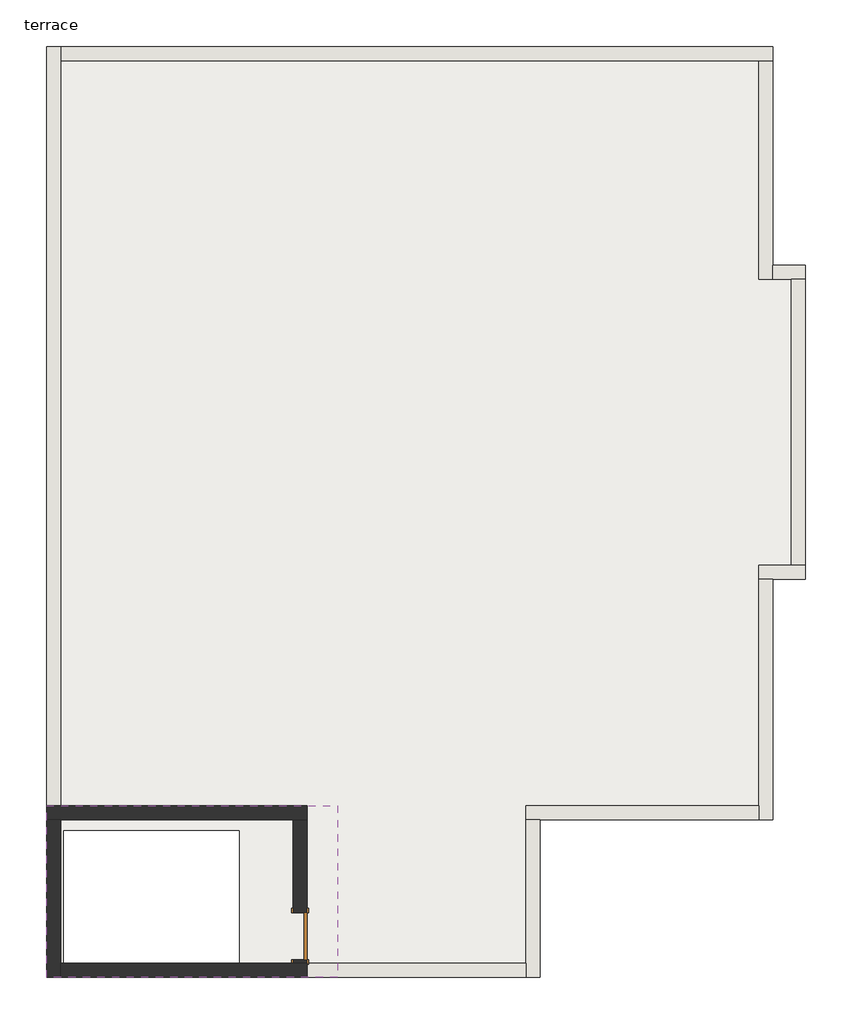
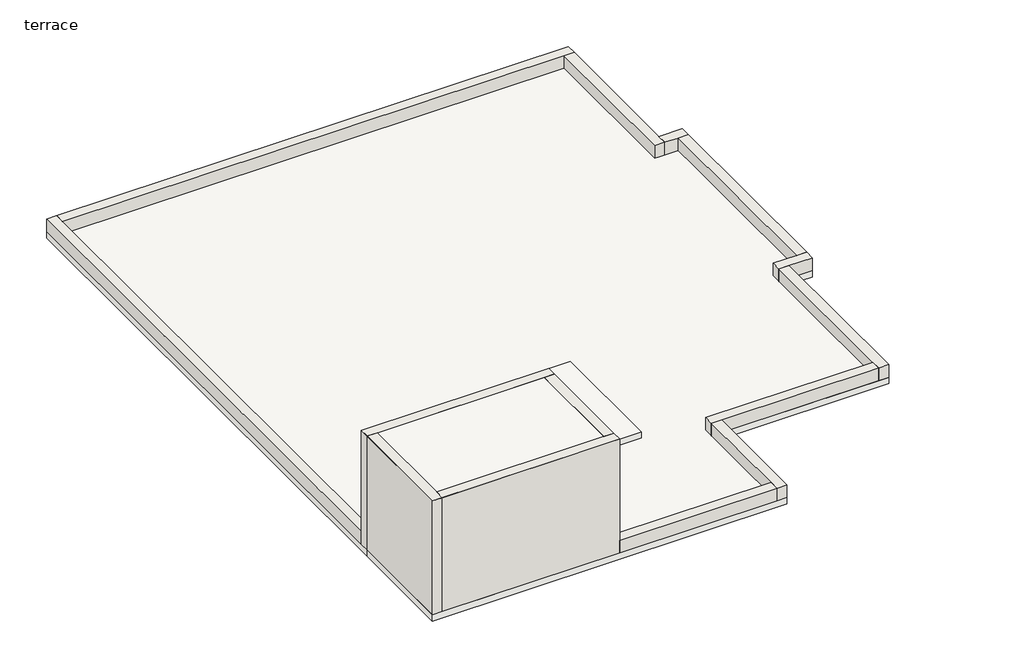
# One storey, incomplete: 14 walls, 2 slabs, 1 door.
"""IFC4 building model written with IfcOpenShell, lengths in millimetres."""

from ifc_helpers import new_model, si_unit, frame, origin, place, context, project, spatial, polyline, outline, extrude, faceted_brep, transform, mapped, element, save
from components import door_bb98abfd

model = new_model("IFC4")

# Units and contexts
model_context = context("Model", 3, world=origin())
ifc_project = project(units=[si_unit("LENGTHUNIT", "METRE", prefix="MILLI")], contexts=[model_context])

# Site, building, storey
site = spatial("IfcSite", under=ifc_project)
building = spatial("IfcBuilding", under=site)
storey = spatial("IfcBuildingStorey", under=building, Name="terrace", Elevation=13411.2)

# Door
placement = place(None, origin())
door_shape = door_bb98abfd(model_context)
element("IfcDoor", 1, ObjectType="Single-Flush : 30\" x 84\"", at=placement, inside=storey, context=model_context, shape_type="MappedRepresentation", body=[
    mapped(door_shape, transform((-9098.9124084, -4373.4038196, 13411.2), x_axis=(0.0, -1.0, 0.0), y_axis=(1.0, 0.0, 0.0), z_axis=(0.0, 0.0, 1.0))),
])

# Slabs
element("IfcSlab", 2, ObjectType="Generic - 6\"", at=placement, inside=storey, context=model_context, shape_type="SweptSolid", body=[
    extrude(outline(polyline([(-1364.6124084, 10180.7961804), (-1364.6124084, 6599.3961804), (-831.2124084, 6599.3961804), (-831.2124084, 1468.5961804), (-1364.6124084, 1468.5961804), (-1364.6124084, -2468.4038196), (-5174.6124084, -2468.4038196), (-5174.6124084, -5046.5038196), (-13251.8124084, -5046.5038196), (-13251.8124084, -2468.4038196), (-13251.8124084, 10180.7961804), (-1364.6124084, 10180.7961804)]), holes=[polyline([(-10102.6120641, -3536.9669819), (-10102.6120641, -2647.9669819), (-12972.8120641, -2647.9669819), (-12972.8120641, -4817.9038196), (-10102.6120641, -4817.9038196), (-10102.6120641, -3536.9669819)])]), frame((0.0, 0.0, 13258.8), z_axis=(0.0, 0.0, 1.0), x_axis=(1.0, 0.0, 0.0)), (0.0, 0.0, 1.0), 152.4),
])
element("IfcSlab", 3, ObjectType="Generic - 6\"", at=placement, inside=storey, context=model_context, shape_type="SweptSolid", body=[
    extrude(outline(polyline([(-8489.3124084, -2239.8038196), (-8489.3124084, -5046.5038196), (-13251.8124084, -5046.5038196), (-13251.8124084, -2239.8038196), (-8489.3124084, -2239.8038196)])), frame((0.0, 0.0, 16002.0), z_axis=(0.0, 0.0, 1.0), x_axis=(1.0, 0.0, 0.0)), (0.0, 0.0, 1.0), 152.4),
])

# Walls
element("IfcWall", 4, ObjectType="Generic - 9\"", at=placement, inside=storey, context=model_context, shape_type="Brep", body=[
    faceted_brep([(-13251.8124084, -2468.4038196, 16154.4), (-13251.8124084, -2468.4038196, 13411.2), (-13251.8124084, -5046.5038196, 13411.2), (-13251.8124084, -5046.5038196, 16154.4), (-13023.2124084, -2468.4038196, 13411.2), (-13023.2124084, -2468.4038196, 16154.4), (-13023.2124084, -4817.9038196, 16154.4), (-13023.2124084, -5046.5038196, 16154.4), (-13023.2124084, -5046.5038196, 13411.2), (-13023.2124084, -4817.9038196, 13411.2)], [[[0, 1, 2, 3]], [[4, 5, 6, 7, 8, 9]], [[2, 1, 4, 9, 8]], [[0, 3, 7, 6, 5]], [[3, 2, 8, 7]], [[0, 5, 4, 1]]]),
])
element("IfcWall", 5, ObjectType="Generic - 9\"", at=placement, inside=storey, context=model_context, shape_type="Brep", body=[
    faceted_brep([(-13023.2124084, -5046.5038196, 13411.2), (-8984.6124084, -5046.5038196, 13411.2), (-8984.6124084, -5046.5038196, 13716.0), (-8984.6124084, -5046.5038196, 16154.4), (-13023.2124084, -5046.5038196, 16154.4), (-13023.2124084, -4817.9038196, 13411.2), (-13023.2124084, -4817.9038196, 16154.4), (-9213.2124084, -4817.9038196, 16154.4), (-8984.6124084, -4817.9038196, 16154.4), (-8984.6124084, -4817.9038196, 13716.0), (-8984.6124084, -4817.9038196, 13411.2), (-9213.2124084, -4817.9038196, 13411.2)], [[[0, 1, 2, 3, 4]], [[5, 6, 7, 8, 9, 10, 11]], [[1, 0, 5, 11, 10]], [[4, 3, 8, 7, 6]], [[0, 4, 6, 5]], [[1, 10, 9, 8, 3, 2]]]),
])
element("IfcWall", 6, ObjectType="Generic - 9\"", at=placement, inside=storey, context=model_context, shape_type="SweptSolid", body=[
    extrude(outline(polyline([(-4754.4038196, 15544.8), (-4754.4038196, 13411.2), (-4817.9038196, 13411.2), (-4817.9038196, 16154.4), (-2468.4038196, 16154.4), (-2468.4038196, 13411.2), (-3992.4038196, 13411.2), (-3992.4038196, 15544.8), (-4754.4038196, 15544.8)])), frame((-9213.2124084, 0.0, 0.0), z_axis=(1.0, 0.0, 0.0), x_axis=(0.0, 1.0, 0.0)), (0.0, 0.0, 1.0), 228.6),
])
element("IfcWall", 7, ObjectType="Generic - 9\"", at=placement, inside=storey, context=model_context, shape_type="Brep", body=[
    faceted_brep([(-13251.8124084, -2468.4038196, 16154.4), (-13251.8124084, -2468.4038196, 13411.2), (-13023.2124084, -2468.4038196, 13411.2), (-9213.2124084, -2468.4038196, 13411.2), (-8984.6124084, -2468.4038196, 13411.2), (-8984.6124084, -2468.4038196, 16154.4), (-9213.2124084, -2468.4038196, 16154.4), (-13023.2124084, -2468.4038196, 16154.4), (-13251.8124084, -2239.8038196, 13411.2), (-13251.8124084, -2239.8038196, 13716.0), (-13251.8124084, -2239.8038196, 16154.4), (-8984.6124084, -2239.8038196, 16154.4), (-8984.6124084, -2239.8038196, 13411.2), (-13023.2124084, -2239.8038196, 13411.2)], [[[0, 1, 2, 3, 4, 5, 6, 7]], [[8, 9, 10, 11, 12, 13]], [[4, 3, 2, 1, 8, 13, 12]], [[0, 7, 6, 5, 11, 10]], [[5, 4, 12, 11]], [[0, 10, 9, 8, 1]]]),
])
element("IfcWall", 8, ObjectType="Generic - 9\"", at=placement, inside=storey, context=model_context, shape_type="Brep", body=[
    faceted_brep([(-13023.2124084, -2239.8038196, 13411.2), (-13023.2124084, 9952.1961804, 13411.2), (-13023.2124084, 10180.7961804, 13411.2), (-13023.2124084, 10180.7961804, 13716.0), (-13023.2124084, 9952.1961804, 13716.0), (-13023.2124084, -2239.8038196, 13716.0), (-13251.8124084, -2239.8038196, 13411.2), (-13251.8124084, -2239.8038196, 13716.0), (-13251.8124084, 10180.7961804, 13716.0), (-13251.8124084, 10180.7961804, 13411.2)], [[[0, 1, 2, 3, 4, 5]], [[6, 7, 8, 9]], [[2, 1, 0, 6, 9]], [[5, 4, 3, 8, 7]], [[0, 5, 7, 6]], [[3, 2, 9, 8]]]),
])
element("IfcWall", 9, ObjectType="Generic - 9\"", at=placement, inside=storey, context=model_context, shape_type="Brep", body=[
    faceted_brep([(-13023.2124084, 9952.1961804, 13411.2), (-1593.2124084, 9952.1961804, 13411.2), (-1364.6124084, 9952.1961804, 13411.2), (-1364.6124084, 9952.1961804, 13716.0), (-1593.2124084, 9952.1961804, 13716.0), (-13023.2124084, 9952.1961804, 13716.0), (-13023.2124084, 10180.7961804, 13411.2), (-13023.2124084, 10180.7961804, 13716.0), (-1364.6124084, 10180.7961804, 13716.0), (-1364.6124084, 10180.7961804, 13411.2)], [[[0, 1, 2, 3, 4, 5]], [[6, 7, 8, 9]], [[2, 1, 0, 6, 9]], [[5, 4, 3, 8, 7]], [[0, 5, 7, 6]], [[3, 2, 9, 8]]]),
])
element("IfcWall", 10, ObjectType="Generic - 9\"", at=placement, inside=storey, context=model_context, shape_type="Brep", body=[
    faceted_brep([(-1593.2124084, 9952.1961804, 13411.2), (-1593.2124084, 6370.7961804, 13411.2), (-1593.2124084, 6370.7961804, 13716.0), (-1593.2124084, 9952.1961804, 13716.0), (-1364.6124084, 9952.1961804, 13411.2), (-1364.6124084, 9952.1961804, 13716.0), (-1364.6124084, 6599.3961804, 13716.0), (-1364.6124084, 6370.7961804, 13716.0), (-1364.6124084, 6370.7961804, 13411.2), (-1364.6124084, 6599.3961804, 13411.2)], [[[0, 1, 2, 3]], [[4, 5, 6, 7, 8, 9]], [[1, 0, 4, 9, 8]], [[3, 2, 7, 6, 5]], [[0, 3, 5, 4]], [[2, 1, 8, 7]]]),
])
element("IfcWall", 11, ObjectType="Generic - 9\"", at=placement, inside=storey, context=model_context, shape_type="Brep", body=[
    faceted_brep([(-1364.6124084, 6370.7961804, 13411.2), (-1059.8124084, 6370.7961804, 13411.2), (-831.2124084, 6370.7961804, 13411.2), (-831.2124084, 6370.7961804, 13716.0), (-1059.8124084, 6370.7961804, 13716.0), (-1364.6124084, 6370.7961804, 13716.0), (-1364.6124084, 6599.3961804, 13411.2), (-1364.6124084, 6599.3961804, 13716.0), (-831.2124084, 6599.3961804, 13716.0), (-831.2124084, 6599.3961804, 13411.2)], [[[0, 1, 2, 3, 4, 5]], [[6, 7, 8, 9]], [[2, 1, 0, 6, 9]], [[5, 4, 3, 8, 7]], [[0, 5, 7, 6]], [[3, 2, 9, 8]]]),
])
element("IfcWall", 12, ObjectType="Generic - 9\"", at=placement, inside=storey, context=model_context, shape_type="SweptSolid", body=[
    extrude(outline(polyline([(-1059.8124084, 1697.1961804), (-1059.8124084, 6370.7961804), (-831.2124084, 6370.7961804), (-831.2124084, 1697.1961804), (-1059.8124084, 1697.1961804)])), frame((0.0, 0.0, 13411.2), z_axis=(0.0, 0.0, 1.0), x_axis=(1.0, 0.0, 0.0)), (0.0, 0.0, 1.0), 304.8),
])
element("IfcWall", 13, ObjectType="Generic - 9\"", at=placement, inside=storey, context=model_context, shape_type="Brep", body=[
    faceted_brep([(-831.2124084, 1697.1961804, 13411.2), (-1059.8124084, 1697.1961804, 13411.2), (-1593.2124084, 1697.1961804, 13411.2), (-1593.2124084, 1697.1961804, 13716.0), (-1059.8124084, 1697.1961804, 13716.0), (-831.2124084, 1697.1961804, 13716.0), (-831.2124084, 1468.5961804, 13411.2), (-831.2124084, 1468.5961804, 13716.0), (-1364.6124084, 1468.5961804, 13716.0), (-1593.2124084, 1468.5961804, 13716.0), (-1593.2124084, 1468.5961804, 13411.2), (-1364.6124084, 1468.5961804, 13411.2)], [[[0, 1, 2, 3, 4, 5]], [[6, 7, 8, 9, 10, 11]], [[2, 1, 0, 6, 11, 10]], [[5, 4, 3, 9, 8, 7]], [[0, 5, 7, 6]], [[3, 2, 10, 9]]]),
])
element("IfcWall", 14, ObjectType="Generic - 9\"", at=placement, inside=storey, context=model_context, shape_type="Brep", body=[
    faceted_brep([(-1593.2124084, 1468.5961804, 13411.2), (-1593.2124084, -2239.8038196, 13411.2), (-1593.2124084, -2468.4038196, 13411.2), (-1593.2124084, -2468.4038196, 13716.0), (-1593.2124084, -2239.8038196, 13716.0), (-1593.2124084, 1468.5961804, 13716.0), (-1364.6124084, 1468.5961804, 13411.2), (-1364.6124084, 1468.5961804, 13716.0), (-1364.6124084, -2468.4038196, 13716.0), (-1364.6124084, -2468.4038196, 13411.2)], [[[0, 1, 2, 3, 4, 5]], [[6, 7, 8, 9]], [[2, 1, 0, 6, 9]], [[5, 4, 3, 8, 7]], [[0, 5, 7, 6]], [[3, 2, 9, 8]]]),
])
element("IfcWall", 15, ObjectType="Generic - 9\"", at=placement, inside=storey, context=model_context, shape_type="Brep", body=[
    faceted_brep([(-1593.2124084, -2239.8038196, 13411.2), (-5403.2124084, -2239.8038196, 13411.2), (-5403.2124084, -2239.8038196, 13716.0), (-1593.2124084, -2239.8038196, 13716.0), (-1593.2124084, -2468.4038196, 13411.2), (-1593.2124084, -2468.4038196, 13716.0), (-5174.6124084, -2468.4038196, 13716.0), (-5403.2124084, -2468.4038196, 13716.0), (-5403.2124084, -2468.4038196, 13411.2), (-5174.6124084, -2468.4038196, 13411.2)], [[[0, 1, 2, 3]], [[4, 5, 6, 7, 8, 9]], [[1, 0, 4, 9, 8]], [[3, 2, 7, 6, 5]], [[0, 3, 5, 4]], [[2, 1, 8, 7]]]),
])
element("IfcWall", 16, ObjectType="Generic - 9\"", at=placement, inside=storey, context=model_context, shape_type="Brep", body=[
    faceted_brep([(-5403.2124084, -2468.4038196, 13411.2), (-5403.2124084, -4817.9038196, 13411.2), (-5403.2124084, -5046.5038196, 13411.2), (-5403.2124084, -5046.5038196, 13716.0), (-5403.2124084, -4817.9038196, 13716.0), (-5403.2124084, -2468.4038196, 13716.0), (-5174.6124084, -2468.4038196, 13411.2), (-5174.6124084, -2468.4038196, 13716.0), (-5174.6124084, -5046.5038196, 13716.0), (-5174.6124084, -5046.5038196, 13411.2)], [[[0, 1, 2, 3, 4, 5]], [[6, 7, 8, 9]], [[2, 1, 0, 6, 9]], [[5, 4, 3, 8, 7]], [[0, 5, 7, 6]], [[3, 2, 9, 8]]]),
])
element("IfcWall", 17, ObjectType="Generic - 9\"", at=placement, inside=storey, context=model_context, shape_type="SweptSolid", body=[
    extrude(outline(polyline([(-8984.6124084, -4817.9038196), (-5403.2124084, -4817.9038196), (-5403.2124084, -5046.5038196), (-8984.6124084, -5046.5038196), (-8984.6124084, -4817.9038196)])), frame((0.0, 0.0, 13411.2), z_axis=(0.0, 0.0, 1.0), x_axis=(1.0, 0.0, 0.0)), (0.0, 0.0, 1.0), 304.8),
])

save(model, "model.ifc")

# Revit data of these elements
# Type "Single-Flush : 30\" x 84\""
#   Type Mark = "4"
#   Construction Type Id = "MDOOR"
#   Assembly Code = "C1020"
#   Analytic Construction = "Metal"
#   Thickness = 0' - 2"
#   Heat Transfer Coefficient (U) = 0.651978 BTU/(h·ft²·°F)
#   Height = 7' - 0"
#   Trim Projection Ext = 0' - 1"
#   Trim Projection Int = 0' - 1"
#   Trim Width = 0' - 3"
#   Width = 2' - 6"
#   Define Thermal Properties by = 1
#   Define Thermal Properties by = 1
#   Door Material = Door - Panel
#   Frame Material = Door - Frame
#   Visual Light Transmittance = 0
#   Solar Heat Gain Coefficient = 0
#   Function = (empty or 0)
#   Wall Closure = (empty or 0)
# Type "Generic - 6\""
#   Assembly Code = "B1010"
#   Function = 0
#   Layers, outside or top first: 0' - 6" no material (function 1)
# Type "Generic - 9\""
#   Assembly Code = "B2010"
#   Layers, outside or top first: 0' - 9" no material (function 1)
# Element 1 (IfcDoor, "Single-Flush : 30\" x 84\"")
#   Phase Created = New Construction
#   Materials on its faces: "Door - Frame", "Door - Panel"
# Element 2 (IfcSlab, "Generic - 6\"")
#   Height Offset From Level = 0' - 0"
#   Phase Created = New Construction
#   Materials on its faces: "Default Floor"
# Element 3 (IfcSlab, "Generic - 6\"")
#   Height Offset From Level = 9' - 0"
#   Phase Created = New Construction
#   Materials on its faces: "Default Floor"
# Elements 4, 5, 6, 7 (IfcWall, "Generic - 9\"")
#   Top Offset = 0' - 0"
#   Base Offset = 0' - 0"
#   Unconnected Height = 9' - 0"
#   wall height = 9' - 0"
#   Phase Created = New Construction
#   Base Constraint = terrace
#   Materials on its faces: "Default Wall"
# Elements 8, 9, 10, 11, 12, 13, 14, 15, 16, 17 (IfcWall, "Generic - 9\"")
#   Top Offset = 0' - 0"
#   Base Offset = 0' - 0"
#   Unconnected Height = 1' - 0"
#   wall height = 1' - 0"
#   Phase Created = New Construction
#   Base Constraint = terrace
#   Materials on its faces: "Default Wall"
# Materials
#   "Door - Panel": class "Wood", colour RGB 210 159 95, transparency 0, Cost = 0
#   "Door - Frame": colour RGB 118 70 51, transparency 0, Cost = 0
#   "Default Floor": colour RGB 128 128 128, transparency 0, Cost = 0
#   "Default Wall": colour RGB 128 128 128, transparency 0, Cost = 0
